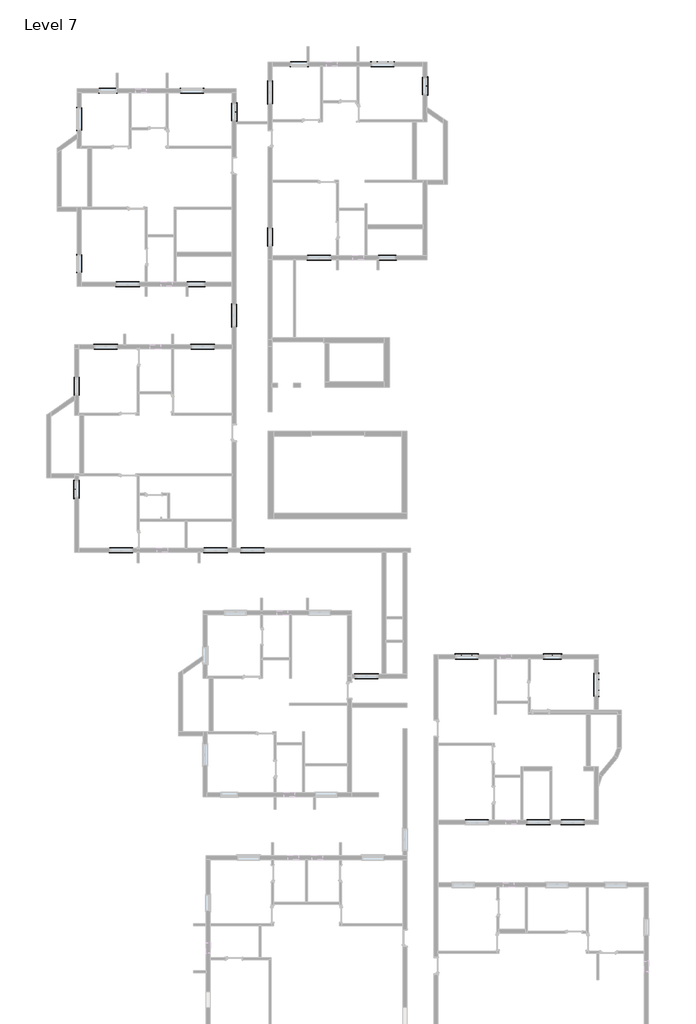
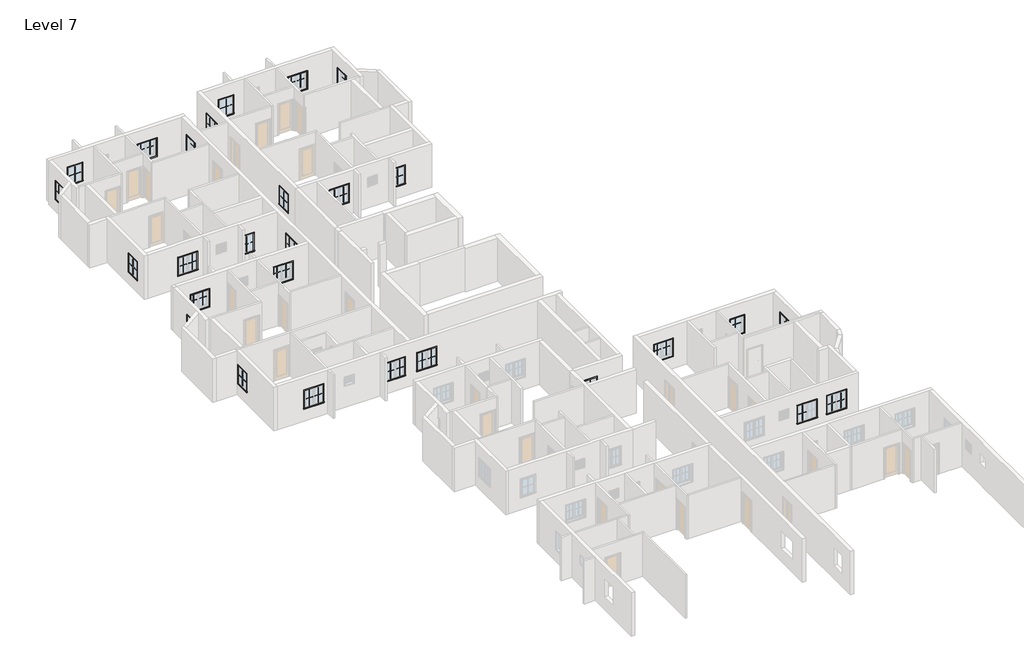
# One storey, part 7 of 7: 101 proxies.
"""IFC4 building model written with IfcOpenShell, lengths in millimetres."""

from ifc_helpers import new_model, si_unit, origin, place, context, project, spatial, transform, mapped, element, save
from components import muntin_pattern_2x2_muntin_pattern_2x2_95b57395, muntin_pattern_2x2_muntin_pattern_2x2_4dfeb3f3, muntin_pattern_2x2_muntin_pattern_2x2_e852a7e4, trim_window_exterior_flat_with_sill_e4b28ec3, trim_window_exterior_flat_with_sill_7cfdd449, trim_window_interior_flat_picture_frame_39ff4276, trim_window_interior_flat_picture_frame_f1e0b15b

model = new_model("IFC4")

# Units and contexts
model_context = context("Model", 3, world=origin())
ifc_project = project(units=[si_unit("LENGTHUNIT", "METRE", prefix="MILLI")], contexts=[model_context])

# Site, building, storey
site = spatial("IfcSite", under=ifc_project)
building = spatial("IfcBuilding", under=site)
storey = spatial("IfcBuildingStorey", under=building, Name="Level 7", Elevation=9601.2)

# Proxies
placement = place(None, origin())
muntin_pattern_2x2_muntin_pattern_2x2_shape = muntin_pattern_2x2_muntin_pattern_2x2_95b57395(model_context)
element("IfcBuildingElementProxy", 1, Name="Muntin Pattern_2x2 : Muntin Pattern_2x2", ObjectType="Muntin Pattern_2x2 : Muntin Pattern_2x2", at=placement, inside=storey, context=model_context, shape_type="MappedRepresentation", body=[
    mapped(muntin_pattern_2x2_muntin_pattern_2x2_shape, transform((-14884.6759469, 4921.5461172, 10585.45), x_axis=(0.0, 1.0, 0.0), y_axis=(-1.0, 0.0, 0.0), z_axis=(0.0, 0.0, 1.0))),
])
element("IfcBuildingElementProxy", 2, Name="Muntin Pattern_2x2 : Muntin Pattern_2x2", ObjectType="Muntin Pattern_2x2 : Muntin Pattern_2x2", at=placement, inside=storey, context=model_context, shape_type="MappedRepresentation", body=[
    mapped(muntin_pattern_2x2_muntin_pattern_2x2_shape, transform((-12990.7362554, 27537.0711172, 10585.45), x_axis=(-1.0, 0.0, 0.0), y_axis=(0.0, -1.0, 0.0), z_axis=(0.0, 0.0, 1.0))),
])
element("IfcBuildingElementProxy", 3, Name="Muntin Pattern_2x2 : Muntin Pattern_2x2", ObjectType="Muntin Pattern_2x2 : Muntin Pattern_2x2", at=placement, inside=storey, context=model_context, shape_type="MappedRepresentation", body=[
    mapped(muntin_pattern_2x2_muntin_pattern_2x2_shape, transform((-5683.5259469, 26431.1755084, 10585.45), x_axis=(0.0, -1.0, 0.0), y_axis=(1.0, 0.0, 0.0), z_axis=(0.0, 0.0, 1.0))),
])
element("IfcBuildingElementProxy", 4, Name="Muntin Pattern_2x2 : Muntin Pattern_2x2", ObjectType="Muntin Pattern_2x2 : Muntin Pattern_2x2", at=placement, inside=storey, context=model_context, shape_type="MappedRepresentation", body=[
    mapped(muntin_pattern_2x2_muntin_pattern_2x2_shape, transform((-7960.0009469, 16513.4711172, 10585.45), x_axis=(-1.0, 0.0, 0.0), y_axis=(0.0, -1.0, 0.0), z_axis=(0.0, 0.0, 1.0))),
])
element("IfcBuildingElementProxy", 5, Name="Muntin Pattern_2x2 : Muntin Pattern_2x2", ObjectType="Muntin Pattern_2x2 : Muntin Pattern_2x2", at=placement, inside=storey, context=model_context, shape_type="MappedRepresentation", body=[
    mapped(muntin_pattern_2x2_muntin_pattern_2x2_shape, transform((-14732.2759469, 17786.6461172, 10585.45), x_axis=(0.0, 1.0, 0.0), y_axis=(-1.0, 0.0, 0.0), z_axis=(0.0, 0.0, 1.0))),
])
element("IfcBuildingElementProxy", 6, Name="Muntin Pattern_2x2 : Muntin Pattern_2x2", ObjectType="Muntin Pattern_2x2 : Muntin Pattern_2x2", at=placement, inside=storey, context=model_context, shape_type="MappedRepresentation", body=[
    mapped(muntin_pattern_2x2_muntin_pattern_2x2_shape, transform((-2075.0862554, 29050.5505084, 10585.45), x_axis=(-1.0, 0.0, 0.0), y_axis=(0.0, -1.0, 0.0), z_axis=(0.0, 0.0, 1.0))),
])
element("IfcBuildingElementProxy", 7, Name="Muntin Pattern_2x2 : Muntin Pattern_2x2", ObjectType="Muntin Pattern_2x2 : Muntin Pattern_2x2", at=placement, inside=storey, context=model_context, shape_type="MappedRepresentation", body=[
    mapped(muntin_pattern_2x2_muntin_pattern_2x2_shape, transform((5213.0740531, 27910.7255084, 10585.45), x_axis=(0.0, -1.0, 0.0), y_axis=(1.0, 0.0, 0.0), z_axis=(0.0, 0.0, 1.0))),
])
element("IfcBuildingElementProxy", 8, Name="Muntin Pattern_2x2 : Muntin Pattern_2x2", ObjectType="Muntin Pattern_2x2 : Muntin Pattern_2x2", at=placement, inside=storey, context=model_context, shape_type="MappedRepresentation", body=[
    mapped(muntin_pattern_2x2_muntin_pattern_2x2_shape, transform((2936.5990531, 18026.9505084, 10585.45), x_axis=(-1.0, 0.0, 0.0), y_axis=(0.0, -1.0, 0.0), z_axis=(0.0, 0.0, 1.0))),
])
element("IfcBuildingElementProxy", 9, Name="Muntin Pattern_2x2 : Muntin Pattern_2x2", ObjectType="Muntin Pattern_2x2 : Muntin Pattern_2x2", at=placement, inside=storey, context=model_context, shape_type="MappedRepresentation", body=[
    mapped(muntin_pattern_2x2_muntin_pattern_2x2_shape, transform((-3835.6759469, 19300.1255084, 10585.45), x_axis=(0.0, 1.0, 0.0), y_axis=(-1.0, 0.0, 0.0), z_axis=(0.0, 0.0, 1.0))),
])
element("IfcBuildingElementProxy", 10, Name="Muntin Pattern_2x2 : Muntin Pattern_2x2", ObjectType="Muntin Pattern_2x2 : Muntin Pattern_2x2", at=placement, inside=storey, context=model_context, shape_type="MappedRepresentation", body=[
    mapped(muntin_pattern_2x2_muntin_pattern_2x2_shape, transform((12366.3490531, -4512.6747229, 10585.45), x_axis=(1.0, 0.0, 0.0), y_axis=(0.0, 1.0, 0.0), z_axis=(0.0, 0.0, 1.0))),
])
element("IfcBuildingElementProxy", 11, Name="Muntin Pattern_2x2 : Muntin Pattern_2x2", ObjectType="Muntin Pattern_2x2 : Muntin Pattern_2x2", at=placement, inside=storey, context=model_context, shape_type="MappedRepresentation", body=[
    mapped(muntin_pattern_2x2_muntin_pattern_2x2_shape, transform((-14675.1259469, 10795.2961172, 10585.45), x_axis=(0.0, -1.0, 0.0), y_axis=(1.0, 0.0, 0.0), z_axis=(0.0, 0.0, 1.0))),
])
muntin_pattern_2x2_muntin_pattern_2x2_2_shape = muntin_pattern_2x2_muntin_pattern_2x2_4dfeb3f3(model_context)
element("IfcBuildingElementProxy", 12, Name="Muntin Pattern_2x2 : Muntin Pattern_2x2", ObjectType="Muntin Pattern_2x2 : Muntin Pattern_2x2", at=placement, inside=storey, context=model_context, shape_type="MappedRepresentation", body=[
    mapped(muntin_pattern_2x2_muntin_pattern_2x2_2_shape, transform((-8498.1634469, 27746.6211172, 10585.45), x_axis=(1.0, 0.0, 0.0), y_axis=(0.0, 1.0, 0.0), z_axis=(0.0, 0.0, 1.0))),
])
element("IfcBuildingElementProxy", 13, Name="Muntin Pattern_2x2 : Muntin Pattern_2x2", ObjectType="Muntin Pattern_2x2 : Muntin Pattern_2x2", at=placement, inside=storey, context=model_context, shape_type="MappedRepresentation", body=[
    mapped(muntin_pattern_2x2_muntin_pattern_2x2_2_shape, transform((-14732.2759469, 25728.9086172, 10585.45), x_axis=(0.0, 1.0, 0.0), y_axis=(-1.0, 0.0, 0.0), z_axis=(0.0, 0.0, 1.0))),
])
element("IfcBuildingElementProxy", 14, Name="Muntin Pattern_2x2 : Muntin Pattern_2x2", ObjectType="Muntin Pattern_2x2 : Muntin Pattern_2x2", at=placement, inside=storey, context=model_context, shape_type="MappedRepresentation", body=[
    mapped(muntin_pattern_2x2_muntin_pattern_2x2_2_shape, transform((-11562.0384469, 16513.4711172, 10585.45), x_axis=(-1.0, 0.0, 0.0), y_axis=(0.0, -1.0, 0.0), z_axis=(0.0, 0.0, 1.0))),
])
element("IfcBuildingElementProxy", 15, Name="Muntin Pattern_2x2 : Muntin Pattern_2x2", ObjectType="Muntin Pattern_2x2 : Muntin Pattern_2x2", at=placement, inside=storey, context=model_context, shape_type="MappedRepresentation", body=[
    mapped(muntin_pattern_2x2_muntin_pattern_2x2_2_shape, transform((-3835.6759469, 27242.3880084, 10585.45), x_axis=(0.0, 1.0, 0.0), y_axis=(-1.0, 0.0, 0.0), z_axis=(0.0, 0.0, 1.0))),
])
element("IfcBuildingElementProxy", 16, Name="Muntin Pattern_2x2 : Muntin Pattern_2x2", ObjectType="Muntin Pattern_2x2 : Muntin Pattern_2x2", at=placement, inside=storey, context=model_context, shape_type="MappedRepresentation", body=[
    mapped(muntin_pattern_2x2_muntin_pattern_2x2_2_shape, transform((2373.0365531, 29260.1005084, 10585.45), x_axis=(1.0, 0.0, 0.0), y_axis=(0.0, 1.0, 0.0), z_axis=(0.0, 0.0, 1.0))),
])
element("IfcBuildingElementProxy", 17, Name="Muntin Pattern_2x2 : Muntin Pattern_2x2", ObjectType="Muntin Pattern_2x2 : Muntin Pattern_2x2", at=placement, inside=storey, context=model_context, shape_type="MappedRepresentation", body=[
    mapped(muntin_pattern_2x2_muntin_pattern_2x2_2_shape, transform((-640.0384469, 18026.9505084, 10585.45), x_axis=(-1.0, 0.0, 0.0), y_axis=(0.0, -1.0, 0.0), z_axis=(0.0, 0.0, 1.0))),
])
element("IfcBuildingElementProxy", 18, Name="Muntin Pattern_2x2 : Muntin Pattern_2x2", ObjectType="Muntin Pattern_2x2 : Muntin Pattern_2x2", at=placement, inside=storey, context=model_context, shape_type="MappedRepresentation", body=[
    mapped(muntin_pattern_2x2_muntin_pattern_2x2_2_shape, transform((14979.3740531, -5923.9622229, 10585.45), x_axis=(0.0, -1.0, 0.0), y_axis=(1.0, 0.0, 0.0), z_axis=(0.0, 0.0, 1.0))),
])
element("IfcBuildingElementProxy", 19, Name="Muntin Pattern_2x2 : Muntin Pattern_2x2", ObjectType="Muntin Pattern_2x2 : Muntin Pattern_2x2", at=placement, inside=storey, context=model_context, shape_type="MappedRepresentation", body=[
    mapped(muntin_pattern_2x2_muntin_pattern_2x2_2_shape, transform((7173.6365531, -4512.6747229, 10585.45), x_axis=(1.0, 0.0, 0.0), y_axis=(0.0, 1.0, 0.0), z_axis=(0.0, 0.0, 1.0))),
])
element("IfcBuildingElementProxy", 20, Name="Muntin Pattern_2x2 : Muntin Pattern_2x2", ObjectType="Muntin Pattern_2x2 : Muntin Pattern_2x2", at=placement, inside=storey, context=model_context, shape_type="MappedRepresentation", body=[
    mapped(muntin_pattern_2x2_muntin_pattern_2x2_2_shape, transform((13825.2615531, -14158.3247229, 10585.45), x_axis=(-1.0, 0.0, 0.0), y_axis=(0.0, -1.0, 0.0), z_axis=(0.0, 0.0, 1.0))),
])
element("IfcBuildingElementProxy", 21, Name="Muntin Pattern_2x2 : Muntin Pattern_2x2", ObjectType="Muntin Pattern_2x2 : Muntin Pattern_2x2", at=placement, inside=storey, context=model_context, shape_type="MappedRepresentation", body=[
    mapped(muntin_pattern_2x2_muntin_pattern_2x2_2_shape, transform((1464.9865531, -5641.6788828, 10585.45), x_axis=(1.0, 0.0, 0.0), y_axis=(0.0, 1.0, 0.0), z_axis=(0.0, 0.0, 1.0))),
])
element("IfcBuildingElementProxy", 22, Name="Muntin Pattern_2x2 : Muntin Pattern_2x2", ObjectType="Muntin Pattern_2x2 : Muntin Pattern_2x2", at=placement, inside=storey, context=model_context, shape_type="MappedRepresentation", body=[
    mapped(muntin_pattern_2x2_muntin_pattern_2x2_2_shape, transform((-4443.6884469, 1349.6711172, 10585.45), x_axis=(-1.0, 0.0, 0.0), y_axis=(0.0, -1.0, 0.0), z_axis=(0.0, 0.0, 1.0))),
])
element("IfcBuildingElementProxy", 23, Name="Muntin Pattern_2x2 : Muntin Pattern_2x2", ObjectType="Muntin Pattern_2x2 : Muntin Pattern_2x2", at=placement, inside=storey, context=model_context, shape_type="MappedRepresentation", body=[
    mapped(muntin_pattern_2x2_muntin_pattern_2x2_2_shape, transform((-6540.8708092, 1349.6711172, 10585.45), x_axis=(-1.0, 0.0, 0.0), y_axis=(0.0, -1.0, 0.0), z_axis=(0.0, 0.0, 1.0))),
])
element("IfcBuildingElementProxy", 24, Name="Muntin Pattern_2x2 : Muntin Pattern_2x2", ObjectType="Muntin Pattern_2x2 : Muntin Pattern_2x2", at=placement, inside=storey, context=model_context, shape_type="MappedRepresentation", body=[
    mapped(muntin_pattern_2x2_muntin_pattern_2x2_2_shape, transform((-11943.0384469, 1349.6711172, 10585.45), x_axis=(-1.0, 0.0, 0.0), y_axis=(0.0, -1.0, 0.0), z_axis=(0.0, 0.0, 1.0))),
])
element("IfcBuildingElementProxy", 25, Name="Muntin Pattern_2x2 : Muntin Pattern_2x2", ObjectType="Muntin Pattern_2x2 : Muntin Pattern_2x2", at=placement, inside=storey, context=model_context, shape_type="MappedRepresentation", body=[
    mapped(muntin_pattern_2x2_muntin_pattern_2x2_2_shape, transform((-13424.2323258, 13141.6211172, 10585.45), x_axis=(1.0, 0.0, 0.0), y_axis=(0.0, 1.0, 0.0), z_axis=(0.0, 0.0, 1.0))),
])
element("IfcBuildingElementProxy", 26, Name="Muntin Pattern_2x2 : Muntin Pattern_2x2", ObjectType="Muntin Pattern_2x2 : Muntin Pattern_2x2", at=placement, inside=storey, context=model_context, shape_type="MappedRepresentation", body=[
    mapped(muntin_pattern_2x2_muntin_pattern_2x2_2_shape, transform((-7888.5634469, 13141.6211172, 10585.45), x_axis=(1.0, 0.0, 0.0), y_axis=(0.0, 1.0, 0.0), z_axis=(0.0, 0.0, 1.0))),
])
element("IfcBuildingElementProxy", 27, Name="Muntin Pattern_2x2 : Muntin Pattern_2x2", ObjectType="Muntin Pattern_2x2 : Muntin Pattern_2x2", at=placement, inside=storey, context=model_context, shape_type="MappedRepresentation", body=[
    mapped(muntin_pattern_2x2_muntin_pattern_2x2_2_shape, transform((-5893.0759469, 14524.3336172, 10585.45), x_axis=(0.0, 1.0, 0.0), y_axis=(-1.0, 0.0, 0.0), z_axis=(0.0, 0.0, 1.0))),
])
muntin_pattern_2x2_muntin_pattern_2x2_3_shape = muntin_pattern_2x2_muntin_pattern_2x2_e852a7e4(model_context)
element("IfcBuildingElementProxy", 28, Name="Muntin Pattern_2x2 : Muntin Pattern_2x2", ObjectType="Muntin Pattern_2x2 : Muntin Pattern_2x2", at=placement, inside=storey, context=model_context, shape_type="MappedRepresentation", body=[
    mapped(muntin_pattern_2x2_muntin_pattern_2x2_3_shape, transform((-7891.7384469, 27746.6211172, 10585.45), x_axis=(-1.0, 0.0, 0.0), y_axis=(0.0, -1.0, 0.0), z_axis=(0.0, 0.0, 1.0))),
])
element("IfcBuildingElementProxy", 29, Name="Muntin Pattern_2x2 : Muntin Pattern_2x2", ObjectType="Muntin Pattern_2x2 : Muntin Pattern_2x2", at=placement, inside=storey, context=model_context, shape_type="MappedRepresentation", body=[
    mapped(muntin_pattern_2x2_muntin_pattern_2x2_3_shape, transform((-14732.2759469, 26335.3336172, 10585.45), x_axis=(0.0, -1.0, 0.0), y_axis=(1.0, 0.0, 0.0), z_axis=(0.0, 0.0, 1.0))),
])
element("IfcBuildingElementProxy", 30, Name="Muntin Pattern_2x2 : Muntin Pattern_2x2", ObjectType="Muntin Pattern_2x2 : Muntin Pattern_2x2", at=placement, inside=storey, context=model_context, shape_type="MappedRepresentation", body=[
    mapped(muntin_pattern_2x2_muntin_pattern_2x2_3_shape, transform((-12168.4634469, 16513.4711172, 10585.45), x_axis=(1.0, 0.0, 0.0), y_axis=(0.0, 1.0, 0.0), z_axis=(0.0, 0.0, 1.0))),
])
element("IfcBuildingElementProxy", 31, Name="Muntin Pattern_2x2 : Muntin Pattern_2x2", ObjectType="Muntin Pattern_2x2 : Muntin Pattern_2x2", at=placement, inside=storey, context=model_context, shape_type="MappedRepresentation", body=[
    mapped(muntin_pattern_2x2_muntin_pattern_2x2_3_shape, transform((-3835.6759469, 27848.8130084, 10585.45), x_axis=(0.0, -1.0, 0.0), y_axis=(1.0, 0.0, 0.0), z_axis=(0.0, 0.0, 1.0))),
])
element("IfcBuildingElementProxy", 32, Name="Muntin Pattern_2x2 : Muntin Pattern_2x2", ObjectType="Muntin Pattern_2x2 : Muntin Pattern_2x2", at=placement, inside=storey, context=model_context, shape_type="MappedRepresentation", body=[
    mapped(muntin_pattern_2x2_muntin_pattern_2x2_3_shape, transform((2979.4615531, 29260.1005084, 10585.45), x_axis=(-1.0, 0.0, 0.0), y_axis=(0.0, -1.0, 0.0), z_axis=(0.0, 0.0, 1.0))),
])
element("IfcBuildingElementProxy", 33, Name="Muntin Pattern_2x2 : Muntin Pattern_2x2", ObjectType="Muntin Pattern_2x2 : Muntin Pattern_2x2", at=placement, inside=storey, context=model_context, shape_type="MappedRepresentation", body=[
    mapped(muntin_pattern_2x2_muntin_pattern_2x2_3_shape, transform((-1246.4634469, 18026.9505084, 10585.45), x_axis=(1.0, 0.0, 0.0), y_axis=(0.0, 1.0, 0.0), z_axis=(0.0, 0.0, 1.0))),
])
element("IfcBuildingElementProxy", 34, Name="Muntin Pattern_2x2 : Muntin Pattern_2x2", ObjectType="Muntin Pattern_2x2 : Muntin Pattern_2x2", at=placement, inside=storey, context=model_context, shape_type="MappedRepresentation", body=[
    mapped(muntin_pattern_2x2_muntin_pattern_2x2_3_shape, transform((14979.3740531, -6530.3872229, 10585.45), x_axis=(0.0, 1.0, 0.0), y_axis=(-1.0, 0.0, 0.0), z_axis=(0.0, 0.0, 1.0))),
])
element("IfcBuildingElementProxy", 35, Name="Muntin Pattern_2x2 : Muntin Pattern_2x2", ObjectType="Muntin Pattern_2x2 : Muntin Pattern_2x2", at=placement, inside=storey, context=model_context, shape_type="MappedRepresentation", body=[
    mapped(muntin_pattern_2x2_muntin_pattern_2x2_3_shape, transform((7780.0615531, -4512.6747229, 10585.45), x_axis=(-1.0, 0.0, 0.0), y_axis=(0.0, -1.0, 0.0), z_axis=(0.0, 0.0, 1.0))),
])
element("IfcBuildingElementProxy", 36, Name="Muntin Pattern_2x2 : Muntin Pattern_2x2", ObjectType="Muntin Pattern_2x2 : Muntin Pattern_2x2", at=placement, inside=storey, context=model_context, shape_type="MappedRepresentation", body=[
    mapped(muntin_pattern_2x2_muntin_pattern_2x2_3_shape, transform((13218.8365531, -14158.3247229, 10585.45), x_axis=(1.0, 0.0, 0.0), y_axis=(0.0, 1.0, 0.0), z_axis=(0.0, 0.0, 1.0))),
])
element("IfcBuildingElementProxy", 37, Name="Muntin Pattern_2x2 : Muntin Pattern_2x2", ObjectType="Muntin Pattern_2x2 : Muntin Pattern_2x2", at=placement, inside=storey, context=model_context, shape_type="MappedRepresentation", body=[
    mapped(muntin_pattern_2x2_muntin_pattern_2x2_3_shape, transform((11263.0365531, -14158.3247229, 10585.45), x_axis=(1.0, 0.0, 0.0), y_axis=(0.0, 1.0, 0.0), z_axis=(0.0, 0.0, 1.0))),
])
element("IfcBuildingElementProxy", 38, Name="Muntin Pattern_2x2 : Muntin Pattern_2x2", ObjectType="Muntin Pattern_2x2 : Muntin Pattern_2x2", at=placement, inside=storey, context=model_context, shape_type="MappedRepresentation", body=[
    mapped(muntin_pattern_2x2_muntin_pattern_2x2_3_shape, transform((2071.4115531, -5641.6788828, 10585.45), x_axis=(-1.0, 0.0, 0.0), y_axis=(0.0, -1.0, 0.0), z_axis=(0.0, 0.0, 1.0))),
])
element("IfcBuildingElementProxy", 39, Name="Muntin Pattern_2x2 : Muntin Pattern_2x2", ObjectType="Muntin Pattern_2x2 : Muntin Pattern_2x2", at=placement, inside=storey, context=model_context, shape_type="MappedRepresentation", body=[
    mapped(muntin_pattern_2x2_muntin_pattern_2x2_3_shape, transform((-5050.1134469, 1349.6711172, 10585.45), x_axis=(1.0, 0.0, 0.0), y_axis=(0.0, 1.0, 0.0), z_axis=(0.0, 0.0, 1.0))),
])
element("IfcBuildingElementProxy", 40, Name="Muntin Pattern_2x2 : Muntin Pattern_2x2", ObjectType="Muntin Pattern_2x2 : Muntin Pattern_2x2", at=placement, inside=storey, context=model_context, shape_type="MappedRepresentation", body=[
    mapped(muntin_pattern_2x2_muntin_pattern_2x2_3_shape, transform((-7147.2958092, 1349.6711172, 10585.45), x_axis=(1.0, 0.0, 0.0), y_axis=(0.0, 1.0, 0.0), z_axis=(0.0, 0.0, 1.0))),
])
element("IfcBuildingElementProxy", 41, Name="Muntin Pattern_2x2 : Muntin Pattern_2x2", ObjectType="Muntin Pattern_2x2 : Muntin Pattern_2x2", at=placement, inside=storey, context=model_context, shape_type="MappedRepresentation", body=[
    mapped(muntin_pattern_2x2_muntin_pattern_2x2_3_shape, transform((-12549.4634469, 1349.6711172, 10585.45), x_axis=(1.0, 0.0, 0.0), y_axis=(0.0, 1.0, 0.0), z_axis=(0.0, 0.0, 1.0))),
])
element("IfcBuildingElementProxy", 42, Name="Muntin Pattern_2x2 : Muntin Pattern_2x2", ObjectType="Muntin Pattern_2x2 : Muntin Pattern_2x2", at=placement, inside=storey, context=model_context, shape_type="MappedRepresentation", body=[
    mapped(muntin_pattern_2x2_muntin_pattern_2x2_3_shape, transform((-12817.8073258, 13141.6211172, 10585.45), x_axis=(-1.0, 0.0, 0.0), y_axis=(0.0, -1.0, 0.0), z_axis=(0.0, 0.0, 1.0))),
])
element("IfcBuildingElementProxy", 43, Name="Muntin Pattern_2x2 : Muntin Pattern_2x2", ObjectType="Muntin Pattern_2x2 : Muntin Pattern_2x2", at=placement, inside=storey, context=model_context, shape_type="MappedRepresentation", body=[
    mapped(muntin_pattern_2x2_muntin_pattern_2x2_3_shape, transform((-7282.1384469, 13141.6211172, 10585.45), x_axis=(-1.0, 0.0, 0.0), y_axis=(0.0, -1.0, 0.0), z_axis=(0.0, 0.0, 1.0))),
])
element("IfcBuildingElementProxy", 44, Name="Muntin Pattern_2x2 : Muntin Pattern_2x2", ObjectType="Muntin Pattern_2x2 : Muntin Pattern_2x2", at=placement, inside=storey, context=model_context, shape_type="MappedRepresentation", body=[
    mapped(muntin_pattern_2x2_muntin_pattern_2x2_3_shape, transform((-5893.0759469, 15130.7586172, 10585.45), x_axis=(0.0, -1.0, 0.0), y_axis=(1.0, 0.0, 0.0), z_axis=(0.0, 0.0, 1.0))),
])
trim_window_exterior_flat_with_sill_shape = trim_window_exterior_flat_with_sill_e4b28ec3(model_context)
element("IfcBuildingElementProxy", 45, Name="Trim-Window-Exterior-Flat : with Sill", ObjectType="Trim-Window-Exterior-Flat : with Sill", at=placement, inside=storey, context=model_context, shape_type="MappedRepresentation", body=[
    mapped(trim_window_exterior_flat_with_sill_shape, transform((-14894.2009469, 4921.5461172, 11734.8), x_axis=(0.0, -1.0, 0.0), y_axis=(0.0, 0.0, 1.0), z_axis=(-1.0, 0.0, 0.0))),
])
element("IfcBuildingElementProxy", 46, Name="Trim-Window-Exterior-Flat : with Sill", ObjectType="Trim-Window-Exterior-Flat : with Sill", at=placement, inside=storey, context=model_context, shape_type="MappedRepresentation", body=[
    mapped(trim_window_exterior_flat_with_sill_shape, transform((-12990.7362554, 27527.5461172, 11734.8), x_axis=(1.0, 0.0, 0.0), y_axis=(0.0, 0.0, 1.0), z_axis=(0.0, -1.0, 0.0))),
])
element("IfcBuildingElementProxy", 47, Name="Trim-Window-Exterior-Flat : with Sill", ObjectType="Trim-Window-Exterior-Flat : with Sill", at=placement, inside=storey, context=model_context, shape_type="MappedRepresentation", body=[
    mapped(trim_window_exterior_flat_with_sill_shape, transform((-5674.0009469, 26431.1755084, 11734.8), x_axis=(0.0, 1.0, 0.0), y_axis=(0.0, 0.0, 1.0), z_axis=(1.0, 0.0, 0.0))),
])
element("IfcBuildingElementProxy", 48, Name="Trim-Window-Exterior-Flat : with Sill", ObjectType="Trim-Window-Exterior-Flat : with Sill", at=placement, inside=storey, context=model_context, shape_type="MappedRepresentation", body=[
    mapped(trim_window_exterior_flat_with_sill_shape, transform((-7960.0009469, 16503.9461172, 11734.8), x_axis=(1.0, 0.0, 0.0), y_axis=(0.0, 0.0, 1.0), z_axis=(0.0, -1.0, 0.0))),
])
element("IfcBuildingElementProxy", 49, Name="Trim-Window-Exterior-Flat : with Sill", ObjectType="Trim-Window-Exterior-Flat : with Sill", at=placement, inside=storey, context=model_context, shape_type="MappedRepresentation", body=[
    mapped(trim_window_exterior_flat_with_sill_shape, transform((-14741.8009469, 17786.6461172, 11734.8), x_axis=(0.0, -1.0, 0.0), y_axis=(0.0, 0.0, 1.0), z_axis=(-1.0, 0.0, 0.0))),
])
element("IfcBuildingElementProxy", 50, Name="Trim-Window-Exterior-Flat : with Sill", ObjectType="Trim-Window-Exterior-Flat : with Sill", at=placement, inside=storey, context=model_context, shape_type="MappedRepresentation", body=[
    mapped(trim_window_exterior_flat_with_sill_shape, transform((-2075.0862554, 29041.0255084, 11734.8), x_axis=(1.0, 0.0, 0.0), y_axis=(0.0, 0.0, 1.0), z_axis=(0.0, -1.0, 0.0))),
])
element("IfcBuildingElementProxy", 51, Name="Trim-Window-Exterior-Flat : with Sill", ObjectType="Trim-Window-Exterior-Flat : with Sill", at=placement, inside=storey, context=model_context, shape_type="MappedRepresentation", body=[
    mapped(trim_window_exterior_flat_with_sill_shape, transform((5222.5990531, 27910.7255084, 11734.8), x_axis=(0.0, 1.0, 0.0), y_axis=(0.0, 0.0, 1.0), z_axis=(1.0, 0.0, 0.0))),
])
element("IfcBuildingElementProxy", 52, Name="Trim-Window-Exterior-Flat : with Sill", ObjectType="Trim-Window-Exterior-Flat : with Sill", at=placement, inside=storey, context=model_context, shape_type="MappedRepresentation", body=[
    mapped(trim_window_exterior_flat_with_sill_shape, transform((2936.5990531, 18017.4255084, 11734.8), x_axis=(1.0, 0.0, 0.0), y_axis=(0.0, 0.0, 1.0), z_axis=(0.0, -1.0, 0.0))),
])
element("IfcBuildingElementProxy", 53, Name="Trim-Window-Exterior-Flat : with Sill", ObjectType="Trim-Window-Exterior-Flat : with Sill", at=placement, inside=storey, context=model_context, shape_type="MappedRepresentation", body=[
    mapped(trim_window_exterior_flat_with_sill_shape, transform((-3845.2009469, 19300.1255084, 11734.8), x_axis=(0.0, -1.0, 0.0), y_axis=(0.0, 0.0, 1.0), z_axis=(-1.0, 0.0, 0.0))),
])
element("IfcBuildingElementProxy", 54, Name="Trim-Window-Exterior-Flat : with Sill", ObjectType="Trim-Window-Exterior-Flat : with Sill", at=placement, inside=storey, context=model_context, shape_type="MappedRepresentation", body=[
    mapped(trim_window_exterior_flat_with_sill_shape, transform((12366.3490531, -4503.1497229, 11734.8), x_axis=(-1.0, 0.0, 0.0), y_axis=(0.0, 0.0, 1.0), z_axis=(0.0, 1.0, 0.0))),
])
element("IfcBuildingElementProxy", 55, Name="Trim-Window-Exterior-Flat : with Sill", ObjectType="Trim-Window-Exterior-Flat : with Sill", at=placement, inside=storey, context=model_context, shape_type="MappedRepresentation", body=[
    mapped(trim_window_exterior_flat_with_sill_shape, transform((-14665.6009469, 10795.2961172, 11734.8), x_axis=(0.0, 1.0, 0.0), y_axis=(0.0, 0.0, 1.0), z_axis=(1.0, 0.0, 0.0))),
])
trim_window_exterior_flat_with_sill_2_shape = trim_window_exterior_flat_with_sill_7cfdd449(model_context)
element("IfcBuildingElementProxy", 56, Name="Trim-Window-Exterior-Flat : with Sill", ObjectType="Trim-Window-Exterior-Flat : with Sill", at=placement, inside=storey, context=model_context, shape_type="MappedRepresentation", body=[
    mapped(trim_window_exterior_flat_with_sill_2_shape, transform((-8194.9509469, 27756.1461172, 11734.8), x_axis=(-1.0, 0.0, 0.0), y_axis=(0.0, 0.0, 1.0), z_axis=(0.0, 1.0, 0.0))),
])
element("IfcBuildingElementProxy", 57, Name="Trim-Window-Exterior-Flat : with Sill", ObjectType="Trim-Window-Exterior-Flat : with Sill", at=placement, inside=storey, context=model_context, shape_type="MappedRepresentation", body=[
    mapped(trim_window_exterior_flat_with_sill_2_shape, transform((-14741.8009469, 26032.1211172, 11734.8), x_axis=(0.0, -1.0, 0.0), y_axis=(0.0, 0.0, 1.0), z_axis=(-1.0, 0.0, 0.0))),
])
element("IfcBuildingElementProxy", 58, Name="Trim-Window-Exterior-Flat : with Sill", ObjectType="Trim-Window-Exterior-Flat : with Sill", at=placement, inside=storey, context=model_context, shape_type="MappedRepresentation", body=[
    mapped(trim_window_exterior_flat_with_sill_2_shape, transform((-11865.2509469, 16503.9461172, 11734.8), x_axis=(1.0, 0.0, 0.0), y_axis=(0.0, 0.0, 1.0), z_axis=(0.0, -1.0, 0.0))),
])
element("IfcBuildingElementProxy", 59, Name="Trim-Window-Exterior-Flat : with Sill", ObjectType="Trim-Window-Exterior-Flat : with Sill", at=placement, inside=storey, context=model_context, shape_type="MappedRepresentation", body=[
    mapped(trim_window_exterior_flat_with_sill_2_shape, transform((-3845.2009469, 27545.6005084, 11734.8), x_axis=(0.0, -1.0, 0.0), y_axis=(0.0, 0.0, 1.0), z_axis=(-1.0, 0.0, 0.0))),
])
element("IfcBuildingElementProxy", 60, Name="Trim-Window-Exterior-Flat : with Sill", ObjectType="Trim-Window-Exterior-Flat : with Sill", at=placement, inside=storey, context=model_context, shape_type="MappedRepresentation", body=[
    mapped(trim_window_exterior_flat_with_sill_2_shape, transform((2676.2490531, 29269.6255084, 11734.8), x_axis=(-1.0, 0.0, 0.0), y_axis=(0.0, 0.0, 1.0), z_axis=(0.0, 1.0, 0.0))),
])
element("IfcBuildingElementProxy", 61, Name="Trim-Window-Exterior-Flat : with Sill", ObjectType="Trim-Window-Exterior-Flat : with Sill", at=placement, inside=storey, context=model_context, shape_type="MappedRepresentation", body=[
    mapped(trim_window_exterior_flat_with_sill_2_shape, transform((-943.2509469, 18017.4255084, 11734.8), x_axis=(1.0, 0.0, 0.0), y_axis=(0.0, 0.0, 1.0), z_axis=(0.0, -1.0, 0.0))),
])
element("IfcBuildingElementProxy", 62, Name="Trim-Window-Exterior-Flat : with Sill", ObjectType="Trim-Window-Exterior-Flat : with Sill", at=placement, inside=storey, context=model_context, shape_type="MappedRepresentation", body=[
    mapped(trim_window_exterior_flat_with_sill_2_shape, transform((14988.8990531, -6227.1747229, 11734.8), x_axis=(0.0, 1.0, 0.0), y_axis=(0.0, 0.0, 1.0), z_axis=(1.0, 0.0, 0.0))),
])
element("IfcBuildingElementProxy", 63, Name="Trim-Window-Exterior-Flat : with Sill", ObjectType="Trim-Window-Exterior-Flat : with Sill", at=placement, inside=storey, context=model_context, shape_type="MappedRepresentation", body=[
    mapped(trim_window_exterior_flat_with_sill_2_shape, transform((7476.8490531, -4503.1497229, 11734.8), x_axis=(-1.0, 0.0, 0.0), y_axis=(0.0, 0.0, 1.0), z_axis=(0.0, 1.0, 0.0))),
])
element("IfcBuildingElementProxy", 64, Name="Trim-Window-Exterior-Flat : with Sill", ObjectType="Trim-Window-Exterior-Flat : with Sill", at=placement, inside=storey, context=model_context, shape_type="MappedRepresentation", body=[
    mapped(trim_window_exterior_flat_with_sill_2_shape, transform((13522.0490531, -14167.8497229, 11734.8), x_axis=(1.0, 0.0, 0.0), y_axis=(0.0, 0.0, 1.0), z_axis=(0.0, -1.0, 0.0))),
])
element("IfcBuildingElementProxy", 65, Name="Trim-Window-Exterior-Flat : with Sill", ObjectType="Trim-Window-Exterior-Flat : with Sill", at=placement, inside=storey, context=model_context, shape_type="MappedRepresentation", body=[
    mapped(trim_window_exterior_flat_with_sill_2_shape, transform((11566.2490531, -14167.8497229, 11734.8), x_axis=(1.0, 0.0, 0.0), y_axis=(0.0, 0.0, 1.0), z_axis=(0.0, -1.0, 0.0))),
])
element("IfcBuildingElementProxy", 66, Name="Trim-Window-Exterior-Flat : with Sill", ObjectType="Trim-Window-Exterior-Flat : with Sill", at=placement, inside=storey, context=model_context, shape_type="MappedRepresentation", body=[
    mapped(trim_window_exterior_flat_with_sill_2_shape, transform((1768.1990531, -5632.1538828, 11734.8), x_axis=(-1.0, 0.0, 0.0), y_axis=(0.0, 0.0, 1.0), z_axis=(0.0, 1.0, 0.0))),
])
element("IfcBuildingElementProxy", 67, Name="Trim-Window-Exterior-Flat : with Sill", ObjectType="Trim-Window-Exterior-Flat : with Sill", at=placement, inside=storey, context=model_context, shape_type="MappedRepresentation", body=[
    mapped(trim_window_exterior_flat_with_sill_2_shape, transform((-4746.9009469, 1340.1461172, 11734.8), x_axis=(1.0, 0.0, 0.0), y_axis=(0.0, 0.0, 1.0), z_axis=(0.0, -1.0, 0.0))),
])
element("IfcBuildingElementProxy", 68, Name="Trim-Window-Exterior-Flat : with Sill", ObjectType="Trim-Window-Exterior-Flat : with Sill", at=placement, inside=storey, context=model_context, shape_type="MappedRepresentation", body=[
    mapped(trim_window_exterior_flat_with_sill_2_shape, transform((-6844.0833092, 1340.1461172, 11734.8), x_axis=(1.0, 0.0, 0.0), y_axis=(0.0, 0.0, 1.0), z_axis=(0.0, -1.0, 0.0))),
])
element("IfcBuildingElementProxy", 69, Name="Trim-Window-Exterior-Flat : with Sill", ObjectType="Trim-Window-Exterior-Flat : with Sill", at=placement, inside=storey, context=model_context, shape_type="MappedRepresentation", body=[
    mapped(trim_window_exterior_flat_with_sill_2_shape, transform((-12246.2509469, 1340.1461172, 11734.8), x_axis=(1.0, 0.0, 0.0), y_axis=(0.0, 0.0, 1.0), z_axis=(0.0, -1.0, 0.0))),
])
element("IfcBuildingElementProxy", 70, Name="Trim-Window-Exterior-Flat : with Sill", ObjectType="Trim-Window-Exterior-Flat : with Sill", at=placement, inside=storey, context=model_context, shape_type="MappedRepresentation", body=[
    mapped(trim_window_exterior_flat_with_sill_2_shape, transform((-13121.0198258, 13151.1461172, 11734.8), x_axis=(-1.0, 0.0, 0.0), y_axis=(0.0, 0.0, 1.0), z_axis=(0.0, 1.0, 0.0))),
])
element("IfcBuildingElementProxy", 71, Name="Trim-Window-Exterior-Flat : with Sill", ObjectType="Trim-Window-Exterior-Flat : with Sill", at=placement, inside=storey, context=model_context, shape_type="MappedRepresentation", body=[
    mapped(trim_window_exterior_flat_with_sill_2_shape, transform((-7585.3509469, 13151.1461172, 11734.8), x_axis=(-1.0, 0.0, 0.0), y_axis=(0.0, 0.0, 1.0), z_axis=(0.0, 1.0, 0.0))),
])
element("IfcBuildingElementProxy", 72, Name="Trim-Window-Exterior-Flat : with Sill", ObjectType="Trim-Window-Exterior-Flat : with Sill", at=placement, inside=storey, context=model_context, shape_type="MappedRepresentation", body=[
    mapped(trim_window_exterior_flat_with_sill_2_shape, transform((-5902.6009469, 14827.5461172, 11734.8), x_axis=(0.0, -1.0, 0.0), y_axis=(0.0, 0.0, 1.0), z_axis=(-1.0, 0.0, 0.0))),
])
trim_window_interior_flat_picture_frame_shape = trim_window_interior_flat_picture_frame_39ff4276(model_context)
element("IfcBuildingElementProxy", 73, Name="Trim-Window-Interior-Flat : Picture Frame", ObjectType="Trim-Window-Interior-Flat : Picture Frame", at=placement, inside=storey, context=model_context, shape_type="MappedRepresentation", body=[
    mapped(trim_window_interior_flat_picture_frame_shape, transform((-14665.6009469, 4921.5461172, 11734.8), x_axis=(0.0, 1.0, 0.0), y_axis=(0.0, 0.0, 1.0), z_axis=(1.0, 0.0, 0.0))),
])
element("IfcBuildingElementProxy", 74, Name="Trim-Window-Interior-Flat : Picture Frame", ObjectType="Trim-Window-Interior-Flat : Picture Frame", at=placement, inside=storey, context=model_context, shape_type="MappedRepresentation", body=[
    mapped(trim_window_interior_flat_picture_frame_shape, transform((-12990.7362554, 27756.1461172, 11734.8), x_axis=(-1.0, 0.0, 0.0), y_axis=(0.0, 0.0, 1.0), z_axis=(0.0, 1.0, 0.0))),
])
element("IfcBuildingElementProxy", 75, Name="Trim-Window-Interior-Flat : Picture Frame", ObjectType="Trim-Window-Interior-Flat : Picture Frame", at=placement, inside=storey, context=model_context, shape_type="MappedRepresentation", body=[
    mapped(trim_window_interior_flat_picture_frame_shape, transform((-5902.6009469, 26431.1755084, 11734.8), x_axis=(0.0, -1.0, 0.0), y_axis=(0.0, 0.0, 1.0), z_axis=(-1.0, 0.0, 0.0))),
])
element("IfcBuildingElementProxy", 76, Name="Trim-Window-Interior-Flat : Picture Frame", ObjectType="Trim-Window-Interior-Flat : Picture Frame", at=placement, inside=storey, context=model_context, shape_type="MappedRepresentation", body=[
    mapped(trim_window_interior_flat_picture_frame_shape, transform((-7960.0009469, 16732.5461172, 11734.8), x_axis=(-1.0, 0.0, 0.0), y_axis=(0.0, 0.0, 1.0), z_axis=(0.0, 1.0, 0.0))),
])
element("IfcBuildingElementProxy", 77, Name="Trim-Window-Interior-Flat : Picture Frame", ObjectType="Trim-Window-Interior-Flat : Picture Frame", at=placement, inside=storey, context=model_context, shape_type="MappedRepresentation", body=[
    mapped(trim_window_interior_flat_picture_frame_shape, transform((-14513.2009469, 17786.6461172, 11734.8), x_axis=(0.0, 1.0, 0.0), y_axis=(0.0, 0.0, 1.0), z_axis=(1.0, 0.0, 0.0))),
])
element("IfcBuildingElementProxy", 78, Name="Trim-Window-Interior-Flat : Picture Frame", ObjectType="Trim-Window-Interior-Flat : Picture Frame", at=placement, inside=storey, context=model_context, shape_type="MappedRepresentation", body=[
    mapped(trim_window_interior_flat_picture_frame_shape, transform((-2075.0862554, 29269.6255084, 11734.8), x_axis=(-1.0, 0.0, 0.0), y_axis=(0.0, 0.0, 1.0), z_axis=(0.0, 1.0, 0.0))),
])
element("IfcBuildingElementProxy", 79, Name="Trim-Window-Interior-Flat : Picture Frame", ObjectType="Trim-Window-Interior-Flat : Picture Frame", at=placement, inside=storey, context=model_context, shape_type="MappedRepresentation", body=[
    mapped(trim_window_interior_flat_picture_frame_shape, transform((4993.9990531, 27910.7255084, 11734.8), x_axis=(0.0, -1.0, 0.0), y_axis=(0.0, 0.0, 1.0), z_axis=(-1.0, 0.0, 0.0))),
])
element("IfcBuildingElementProxy", 80, Name="Trim-Window-Interior-Flat : Picture Frame", ObjectType="Trim-Window-Interior-Flat : Picture Frame", at=placement, inside=storey, context=model_context, shape_type="MappedRepresentation", body=[
    mapped(trim_window_interior_flat_picture_frame_shape, transform((2936.5990531, 18246.0255084, 11734.8), x_axis=(-1.0, 0.0, 0.0), y_axis=(0.0, 0.0, 1.0), z_axis=(0.0, 1.0, 0.0))),
])
element("IfcBuildingElementProxy", 81, Name="Trim-Window-Interior-Flat : Picture Frame", ObjectType="Trim-Window-Interior-Flat : Picture Frame", at=placement, inside=storey, context=model_context, shape_type="MappedRepresentation", body=[
    mapped(trim_window_interior_flat_picture_frame_shape, transform((-3616.6009469, 19300.1255084, 11734.8), x_axis=(0.0, 1.0, 0.0), y_axis=(0.0, 0.0, 1.0), z_axis=(1.0, 0.0, 0.0))),
])
element("IfcBuildingElementProxy", 82, Name="Trim-Window-Interior-Flat : Picture Frame", ObjectType="Trim-Window-Interior-Flat : Picture Frame", at=placement, inside=storey, context=model_context, shape_type="MappedRepresentation", body=[
    mapped(trim_window_interior_flat_picture_frame_shape, transform((12366.3490531, -4731.7497229, 11734.8), x_axis=(1.0, 0.0, 0.0), y_axis=(0.0, 0.0, 1.0), z_axis=(0.0, -1.0, 0.0))),
])
element("IfcBuildingElementProxy", 83, Name="Trim-Window-Interior-Flat : Picture Frame", ObjectType="Trim-Window-Interior-Flat : Picture Frame", at=placement, inside=storey, context=model_context, shape_type="MappedRepresentation", body=[
    mapped(trim_window_interior_flat_picture_frame_shape, transform((-14894.2009469, 10795.2961172, 11734.8), x_axis=(0.0, -1.0, 0.0), y_axis=(0.0, 0.0, 1.0), z_axis=(-1.0, 0.0, 0.0))),
])
trim_window_interior_flat_picture_frame_2_shape = trim_window_interior_flat_picture_frame_f1e0b15b(model_context)
element("IfcBuildingElementProxy", 84, Name="Trim-Window-Interior-Flat : Picture Frame", ObjectType="Trim-Window-Interior-Flat : Picture Frame", at=placement, inside=storey, context=model_context, shape_type="MappedRepresentation", body=[
    mapped(trim_window_interior_flat_picture_frame_2_shape, transform((-8194.9509469, 27527.5461172, 11734.8), x_axis=(1.0, 0.0, 0.0), y_axis=(0.0, 0.0, 1.0), z_axis=(0.0, -1.0, 0.0))),
])
element("IfcBuildingElementProxy", 85, Name="Trim-Window-Interior-Flat : Picture Frame", ObjectType="Trim-Window-Interior-Flat : Picture Frame", at=placement, inside=storey, context=model_context, shape_type="MappedRepresentation", body=[
    mapped(trim_window_interior_flat_picture_frame_2_shape, transform((-14513.2009469, 26032.1211172, 11734.8), x_axis=(0.0, 1.0, 0.0), y_axis=(0.0, 0.0, 1.0), z_axis=(1.0, 0.0, 0.0))),
])
element("IfcBuildingElementProxy", 86, Name="Trim-Window-Interior-Flat : Picture Frame", ObjectType="Trim-Window-Interior-Flat : Picture Frame", at=placement, inside=storey, context=model_context, shape_type="MappedRepresentation", body=[
    mapped(trim_window_interior_flat_picture_frame_2_shape, transform((-11865.2509469, 16732.5461172, 11734.8), x_axis=(-1.0, 0.0, 0.0), y_axis=(0.0, 0.0, 1.0), z_axis=(0.0, 1.0, 0.0))),
])
element("IfcBuildingElementProxy", 87, Name="Trim-Window-Interior-Flat : Picture Frame", ObjectType="Trim-Window-Interior-Flat : Picture Frame", at=placement, inside=storey, context=model_context, shape_type="MappedRepresentation", body=[
    mapped(trim_window_interior_flat_picture_frame_2_shape, transform((-3616.6009469, 27545.6005084, 11734.8), x_axis=(0.0, 1.0, 0.0), y_axis=(0.0, 0.0, 1.0), z_axis=(1.0, 0.0, 0.0))),
])
element("IfcBuildingElementProxy", 88, Name="Trim-Window-Interior-Flat : Picture Frame", ObjectType="Trim-Window-Interior-Flat : Picture Frame", at=placement, inside=storey, context=model_context, shape_type="MappedRepresentation", body=[
    mapped(trim_window_interior_flat_picture_frame_2_shape, transform((2676.2490531, 29041.0255084, 11734.8), x_axis=(1.0, 0.0, 0.0), y_axis=(0.0, 0.0, 1.0), z_axis=(0.0, -1.0, 0.0))),
])
element("IfcBuildingElementProxy", 89, Name="Trim-Window-Interior-Flat : Picture Frame", ObjectType="Trim-Window-Interior-Flat : Picture Frame", at=placement, inside=storey, context=model_context, shape_type="MappedRepresentation", body=[
    mapped(trim_window_interior_flat_picture_frame_2_shape, transform((-943.2509469, 18246.0255084, 11734.8), x_axis=(-1.0, 0.0, 0.0), y_axis=(0.0, 0.0, 1.0), z_axis=(0.0, 1.0, 0.0))),
])
element("IfcBuildingElementProxy", 90, Name="Trim-Window-Interior-Flat : Picture Frame", ObjectType="Trim-Window-Interior-Flat : Picture Frame", at=placement, inside=storey, context=model_context, shape_type="MappedRepresentation", body=[
    mapped(trim_window_interior_flat_picture_frame_2_shape, transform((14760.2990531, -6227.1747229, 11734.8), x_axis=(0.0, -1.0, 0.0), y_axis=(0.0, 0.0, 1.0), z_axis=(-1.0, 0.0, 0.0))),
])
element("IfcBuildingElementProxy", 91, Name="Trim-Window-Interior-Flat : Picture Frame", ObjectType="Trim-Window-Interior-Flat : Picture Frame", at=placement, inside=storey, context=model_context, shape_type="MappedRepresentation", body=[
    mapped(trim_window_interior_flat_picture_frame_2_shape, transform((7476.8490531, -4731.7497229, 11734.8), x_axis=(1.0, 0.0, 0.0), y_axis=(0.0, 0.0, 1.0), z_axis=(0.0, -1.0, 0.0))),
])
element("IfcBuildingElementProxy", 92, Name="Trim-Window-Interior-Flat : Picture Frame", ObjectType="Trim-Window-Interior-Flat : Picture Frame", at=placement, inside=storey, context=model_context, shape_type="MappedRepresentation", body=[
    mapped(trim_window_interior_flat_picture_frame_2_shape, transform((13522.0490531, -13939.2497229, 11734.8), x_axis=(-1.0, 0.0, 0.0), y_axis=(0.0, 0.0, 1.0), z_axis=(0.0, 1.0, 0.0))),
])
element("IfcBuildingElementProxy", 93, Name="Trim-Window-Interior-Flat : Picture Frame", ObjectType="Trim-Window-Interior-Flat : Picture Frame", at=placement, inside=storey, context=model_context, shape_type="MappedRepresentation", body=[
    mapped(trim_window_interior_flat_picture_frame_2_shape, transform((11566.2490531, -13939.2497229, 11734.8), x_axis=(-1.0, 0.0, 0.0), y_axis=(0.0, 0.0, 1.0), z_axis=(0.0, 1.0, 0.0))),
])
element("IfcBuildingElementProxy", 94, Name="Trim-Window-Interior-Flat : Picture Frame", ObjectType="Trim-Window-Interior-Flat : Picture Frame", at=placement, inside=storey, context=model_context, shape_type="MappedRepresentation", body=[
    mapped(trim_window_interior_flat_picture_frame_2_shape, transform((8061.0490531, -13939.2497229, 11734.8), x_axis=(-1.0, 0.0, 0.0), y_axis=(0.0, 0.0, 1.0), z_axis=(0.0, 1.0, 0.0))),
])
element("IfcBuildingElementProxy", 95, Name="Trim-Window-Interior-Flat : Picture Frame", ObjectType="Trim-Window-Interior-Flat : Picture Frame", at=placement, inside=storey, context=model_context, shape_type="MappedRepresentation", body=[
    mapped(trim_window_interior_flat_picture_frame_2_shape, transform((1768.1990531, -5860.7538828, 11734.8), x_axis=(1.0, 0.0, 0.0), y_axis=(0.0, 0.0, 1.0), z_axis=(0.0, -1.0, 0.0))),
])
element("IfcBuildingElementProxy", 96, Name="Trim-Window-Interior-Flat : Picture Frame", ObjectType="Trim-Window-Interior-Flat : Picture Frame", at=placement, inside=storey, context=model_context, shape_type="MappedRepresentation", body=[
    mapped(trim_window_interior_flat_picture_frame_2_shape, transform((-4746.9009469, 1568.7461172, 11734.8), x_axis=(-1.0, 0.0, 0.0), y_axis=(0.0, 0.0, 1.0), z_axis=(0.0, 1.0, 0.0))),
])
element("IfcBuildingElementProxy", 97, Name="Trim-Window-Interior-Flat : Picture Frame", ObjectType="Trim-Window-Interior-Flat : Picture Frame", at=placement, inside=storey, context=model_context, shape_type="MappedRepresentation", body=[
    mapped(trim_window_interior_flat_picture_frame_2_shape, transform((-6844.0833092, 1568.7461172, 11734.8), x_axis=(-1.0, 0.0, 0.0), y_axis=(0.0, 0.0, 1.0), z_axis=(0.0, 1.0, 0.0))),
])
element("IfcBuildingElementProxy", 98, Name="Trim-Window-Interior-Flat : Picture Frame", ObjectType="Trim-Window-Interior-Flat : Picture Frame", at=placement, inside=storey, context=model_context, shape_type="MappedRepresentation", body=[
    mapped(trim_window_interior_flat_picture_frame_2_shape, transform((-12246.2509469, 1568.7461172, 11734.8), x_axis=(-1.0, 0.0, 0.0), y_axis=(0.0, 0.0, 1.0), z_axis=(0.0, 1.0, 0.0))),
])
element("IfcBuildingElementProxy", 99, Name="Trim-Window-Interior-Flat : Picture Frame", ObjectType="Trim-Window-Interior-Flat : Picture Frame", at=placement, inside=storey, context=model_context, shape_type="MappedRepresentation", body=[
    mapped(trim_window_interior_flat_picture_frame_2_shape, transform((-13121.0198258, 12922.5461172, 11734.8), x_axis=(1.0, 0.0, 0.0), y_axis=(0.0, 0.0, 1.0), z_axis=(0.0, -1.0, 0.0))),
])
element("IfcBuildingElementProxy", 100, Name="Trim-Window-Interior-Flat : Picture Frame", ObjectType="Trim-Window-Interior-Flat : Picture Frame", at=placement, inside=storey, context=model_context, shape_type="MappedRepresentation", body=[
    mapped(trim_window_interior_flat_picture_frame_2_shape, transform((-7585.3509469, 12922.5461172, 11734.8), x_axis=(1.0, 0.0, 0.0), y_axis=(0.0, 0.0, 1.0), z_axis=(0.0, -1.0, 0.0))),
])
element("IfcBuildingElementProxy", 101, Name="Trim-Window-Interior-Flat : Picture Frame", ObjectType="Trim-Window-Interior-Flat : Picture Frame", at=placement, inside=storey, context=model_context, shape_type="MappedRepresentation", body=[
    mapped(trim_window_interior_flat_picture_frame_2_shape, transform((-5674.0009469, 14827.5461172, 11734.8), x_axis=(0.0, 1.0, 0.0), y_axis=(0.0, 0.0, 1.0), z_axis=(1.0, 0.0, 0.0))),
])

save(model, "model.ifc")

# Revit data of these elements
# Type "Muntin Pattern_2x2 : Muntin Pattern_2x2"
#   Width [instance default] = 4' - 0"
#   Thickness = 0' - 0 1/2"
#   Height [instance default] = 4' - 0"
#   Distance = 0' - 0 3/4"
#   Interior Material [instance default] = none
#   Exterior Material [instance default] = none
#   Default Elevation = 0
# Type "Trim-Window-Exterior-Flat : with Sill"
#   Trim Width = 0' - 2 1/4"
#   Trim Thickness_Picture Frame = 0' - 1 1/4"
#   Trim Thickness_with Sill = 0' - 0 3/4"
#   Sill Thickness = 0' - 1 1/4"
#   Opening Width [instance default] = 2' - 0"
#   Opening Height [instance default] = 3' - 0"
#   Default Elevation = 4' - 0"
#   Sill = yes
#   Picture Frame = no
#   Trim Material [instance default] = none
# Type "Trim-Window-Interior-Flat : Picture Frame"
#   Trim Thickness_Picture Frame = 0' - 1 1/4"
#   Trim Width = 0' - 2 1/4"
#   Trim Thickness_with Sill = 0' - 0 3/4"
#   Sill Thickness = 0' - 1 1/4"
#   Opening Width [instance default] = 2' - 0"
#   Opening Height [instance default] = 3' - 0"
#   Default Elevation = 4' - 0"
#   Sill = no
#   Picture Frame = yes
#   Trim Material [instance default] = none
# Elements 1, 2, 3, 4, 5, 6, 7, 8, 9, 10, 11 (IfcBuildingElementProxy, "Muntin Pattern_2x2 : Muntin Pattern_2x2")
#   Width = 2' - 6 1/2"
#   Height = 3' - 6 1/2"
#   Interior Material = Wood - Stained
#   Exterior Material = Clad - White
#   Phase Created = New Construction
#   Materials on its faces: "Clad - White", "Wood - Stained"
# Elements 12, 13, 14, 15, 16, 17, 18, 19, 20, 21, 22, 23, 24, 25, 26, 27, 28, 29, 30, 31, 32, 33, 34, 35, 36, 37, 38, 39, 40, 41, 42, 43, 44 (IfcBuildingElementProxy, "Muntin Pattern_2x2 : Muntin Pattern_2x2")
#   Width = 1' - 6 5/8"
#   Height = 3' - 6 1/2"
#   Interior Material = Wood - Stained
#   Exterior Material = Clad - White
#   Phase Created = New Construction
#   Materials on its faces: "Clad - White", "Wood - Stained"
# Elements 45, 46, 47, 48, 49, 50, 51, 52, 53, 54, 55 (IfcBuildingElementProxy, "Trim-Window-Exterior-Flat : with Sill")
#   Opening Width = 3' - 0"
#   Opening Height = 4' - 0"
#   Trim Material = Clad - White
#   Phase Created = New Construction
#   Materials on its faces: "Clad - White"
# Elements 56, 57, 58, 59, 60, 61, 62, 63, 64, 65, 66, 67, 68, 69, 70, 71, 72 (IfcBuildingElementProxy, "Trim-Window-Exterior-Flat : with Sill")
#   Opening Width = 4' - 0"
#   Opening Height = 4' - 0"
#   Trim Material = Clad - White
#   Phase Created = New Construction
#   Materials on its faces: "Clad - White"
# Elements 73, 74, 75, 76, 77, 78, 79, 80, 81, 82, 83 (IfcBuildingElementProxy, "Trim-Window-Interior-Flat : Picture Frame")
#   Opening Width = 3' - 0"
#   Opening Height = 4' - 0"
#   Trim Material = Wood - Stained
#   Phase Created = New Construction
#   Materials on its faces: "Wood - Stained"
# Elements 84, 85, 86, 87, 88, 89, 90, 91, 92, 93, 94, 95, 96, 97, 98, 99, 100, 101 (IfcBuildingElementProxy, "Trim-Window-Interior-Flat : Picture Frame")
#   Opening Width = 4' - 0"
#   Opening Height = 4' - 0"
#   Trim Material = Wood - Stained
#   Phase Created = New Construction
#   Materials on its faces: "Wood - Stained"
# Materials
#   "Clad - White": class "Wood", colour RGB 242 242 238, transparency 0, Cost = 0
#   "Wood - Stained": class "Wood", colour RGB 224 178 126, transparency 0, Cost = 0
